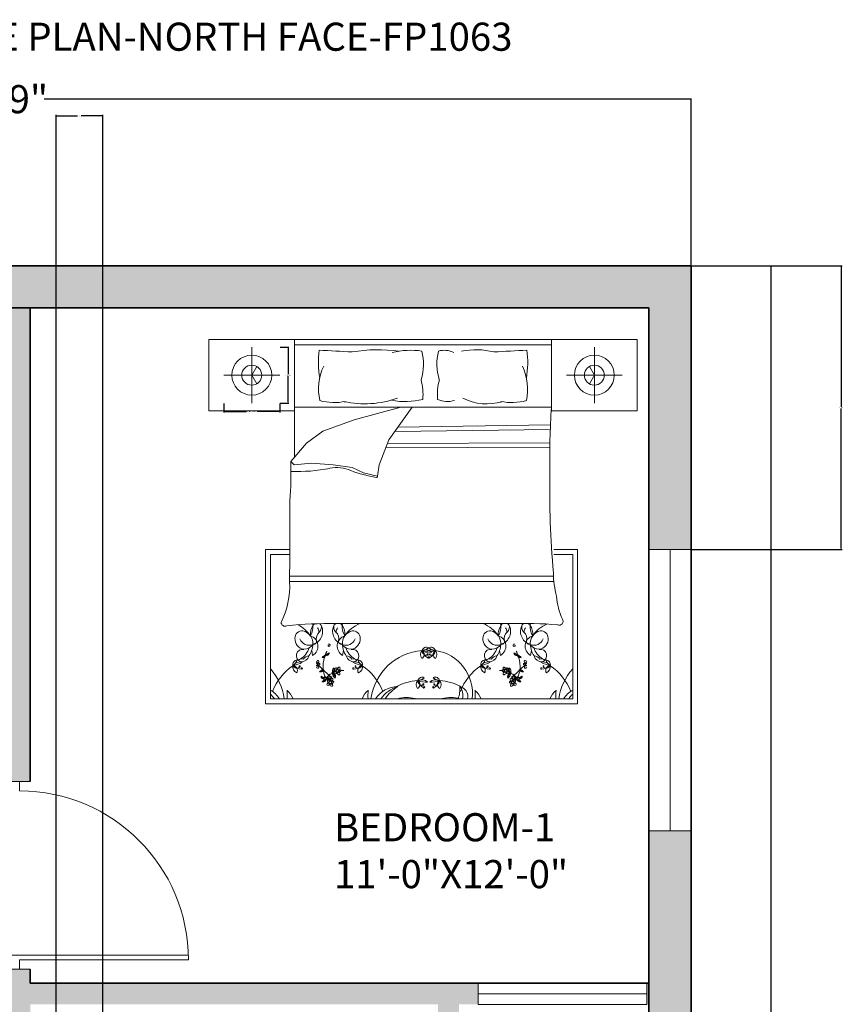
# Model space of a CAD drawing. Units: inches. Extents: x -13 to 349, y -556 to 61.
# Tile 6 of 6: x 174 to 349, y -149 to 61. Entities that reach past the tile are written whole.
import ezdxf

# ---------------------------------------------------------------- set-up
doc = ezdxf.new("R2010")
doc.units = ezdxf.units.IN
doc.header["$MEASUREMENT"] = 0
for name, color, linetype, lineweight in [('A-ANNO-DIMS', 2, 'Continuous', 18), ('A-ANNO-TEXT', 7, 'Continuous', 25), ('A-AREA-IDEN', 7, 'Continuous', 18), ('A-DOOR', 3, 'Continuous', 20), ('A-FURN', 8, 'Continuous', 13), ('A-GLAZ', 5, 'Continuous', 18), ('A-WALL', 7, 'Continuous', 35), ('A-WALL-PATT', 8, 'Continuous', 13)]:
    doc.layers.add(name, color=color, linetype=linetype, lineweight=lineweight)
doc.styles.get("Standard").update_dxf_attribs({"font": 'arial.ttf'})
doc.dimstyles.get("Standard").update_dxf_attribs({"dimtxt": 0.18, "dimasz": 0.18, "dimexe": 0.18, "dimexo": 0.0625, "dimgap": 0.09, "dimtad": 0, "dimtih": 1, "dimtoh": 1, "dimdec": 0, "dimzin": 0, "dimdsep": 46, "dimlunit": 3, "dimtxsty": 'Standard', "dimcen": 0.09, "dimadec": 0, "dimazin": 0, "dimtfac": 1, "dimtdec": 0, "dimtofl": 0, "dimtmove": 0, "dimatfit": 3, "dimfxl": 1, "dimtolj": 1, "dimtzin": 0, "dimarcsym": 0})

# ---------------------------------------------------------------- blocks, each defined once
blk = doc.blocks.new('*D2')
at = {"layer": 'A-ANNO-DIMS', "color": 0, "lineweight": -2, "transparency": 16777216}
for p, q in [((19.76, 8.35), (19.76, 44)), ((19.94, 43.82), (157.81, 43.82)), ((316.58, 43.82), (178.7, 43.82)), ((316.76, 8.35), (316.76, 44))]:
    blk.add_line(p, q, dxfattribs=at)
at = {"layer": 'A-ANNO-DIMS', "color": 0, "transparency": 16777216}
for points in [[(19.94, 43.85), (19.94, 43.79), (19.76, 43.82)], [(316.58, 43.85), (316.58, 43.79), (316.76, 43.82)]]:
    blk.add_solid(points, dxfattribs=at)
at = {"layer": 'Defpoints', "color": 0, "transparency": 16777216}
for p in [(316.76, 43.82), (19.76, 8.29), (316.76, 8.29)]:
    blk.add_point(p, dxfattribs=at)
at = {"layer": 'A-ANNO-DIMS', "color": 0, "transparency": 16777216, "insert": (168.26, 43.82), "char_height": 6, "attachment_point": 5}
blk.add_mtext('\\A1;24\'-9"', dxfattribs=at)
blk = doc.blocks.new('*D3')
at = {"layer": 'A-ANNO-DIMS', "color": 0, "lineweight": -2, "transparency": 16777216}
for p, q in [((316.82, 8.29), (333.9, 8.29)), ((333.72, 8.11), (333.72, -254.62)), ((333.72, -523.53), (333.72, -260.8)), ((316.82, -523.71), (333.9, -523.71))]:
    blk.add_line(p, q, dxfattribs=at)
at = {"layer": 'A-ANNO-DIMS', "color": 0, "transparency": 16777216}
for points in [[(333.69, 8.11), (333.75, 8.11), (333.72, 8.29)], [(333.69, -523.53), (333.75, -523.53), (333.72, -523.71)]]:
    blk.add_solid(points, dxfattribs=at)
at = {"layer": 'Defpoints', "color": 0, "transparency": 16777216}
for p in [(316.76, 8.29), (316.76, -523.71), (333.72, -523.71)]:
    blk.add_point(p, dxfattribs=at)
at = {"layer": 'A-ANNO-DIMS', "color": 0, "transparency": 16777216, "insert": (333.72, -257.71), "char_height": 6, "attachment_point": 5}
blk.add_mtext('\\A1;44\'-4"', dxfattribs=at)
blk = doc.blocks.new('DOOR-SWING-36IN')
for p, q in [((36, 40), (33.75, 40)), ((36, 38), (36, 40)), ((36, 40), (38.25, 40)), ((38.25, 3), (0, 3)), ((36, 2), (0, 2)), ((36, 0), (36, 2)), ((33.75, 0), (38.25, 0))]:
    blk.add_line(p, q)
blk.add_arc((36, 2), 36, 90, 180)
blk = doc.blocks.new('WIN-60IN-D9')
for p, q in [((0, 60), (0, 0)), ((9, 60), (0, 60)), ((4.5, 60), (4.5, 0)), ((9, 0), (9, 60)), ((0, 0), (9, 0))]:
    blk.add_line(p, q)
blk = doc.blocks.new('WIN-36IN-D4_5')
for p, q in [((0, 4.5), (36, 4.5)), ((0, 0), (0, 4.5)), ((36, 4.5), (36, 0)), ((0, 2.25), (36, 2.25)), ((36, 0), (0, 0))]:
    blk.add_line(p, q)
blk = doc.blocks.new('BEDSIDE-LAMP-LG')
for p, q in [((5.97, 0), (5.97, 11.94)), ((0, 5.97), (11.94, 5.97))]:
    blk.add_line(p, q)
for points in [[(5.97, 5.97), (4.91, 7.81)], [(5.97, 5.97), (4.91, 4.12)]]:
    blk.add_lwpolyline(points)
for radius in [4.26, 2.13]:
    blk.add_circle((5.97, 5.97), radius)
blk = doc.blocks.new('*D30')
at = {"layer": 'A-ANNO-DIMS', "color": 0, "lineweight": -2, "transparency": 16777216}
for p, q in [((217.05, -21.06), (217.05, -22.97)), ((217.23, -22.79), (221.89, -22.79)), ((228.81, -22.79), (224.15, -22.79)), ((228.99, -21.06), (228.99, -22.97))]:
    blk.add_line(p, q, dxfattribs=at)
at = {"layer": 'A-ANNO-DIMS', "color": 0, "transparency": 16777216}
for points in [[(217.23, -22.76), (217.23, -22.82), (217.05, -22.79)], [(228.81, -22.76), (228.81, -22.82), (228.99, -22.79)]]:
    blk.add_solid(points, dxfattribs=at)
at = {"layer": 'Defpoints', "color": 0, "transparency": 16777216}
for p in [(217.05, -21), (217.05, -22.79), (228.99, -21)]:
    blk.add_point(p, dxfattribs=at)
at = {"layer": 'A-ANNO-DIMS', "color": 0, "transparency": 16777216, "insert": (223.02, -22.79), "char_height": 0.18, "attachment_point": 5}
blk.add_mtext('\\A1;LAMP A 1\'-0" TYP.', dxfattribs=at)
blk = doc.blocks.new('*D31')
at = {"layer": 'A-ANNO-DIMS', "color": 0, "lineweight": -2, "transparency": 16777216}
for p, q in [((229.05, -9.06), (230.96, -9.06)), ((230.78, -9.24), (230.78, -14.85)), ((230.78, -20.82), (230.78, -15.21)), ((229.05, -21), (230.96, -21))]:
    blk.add_line(p, q, dxfattribs=at)
at = {"layer": 'A-ANNO-DIMS', "color": 0, "transparency": 16777216}
for points in [[(230.75, -9.24), (230.81, -9.24), (230.78, -9.06)], [(230.75, -20.82), (230.81, -20.82), (230.78, -21)]]:
    blk.add_solid(points, dxfattribs=at)
at = {"layer": 'Defpoints', "color": 0, "transparency": 16777216}
for p in [(228.99, -9.06), (228.99, -21), (230.78, -21)]:
    blk.add_point(p, dxfattribs=at)
at = {"layer": 'A-ANNO-DIMS', "color": 0, "transparency": 16777216, "insert": (230.78, -15.03), "char_height": 0.18, "attachment_point": 5}
blk.add_mtext('\\A1;1\'-0" TYP.', dxfattribs=at)
blk = doc.blocks.new('*D37')
at = {"layer": 'A-ANNO-DIMS', "color": 0, "lineweight": -2, "transparency": 16777216}
for p, q in [((181.26, -353.65), (181.26, 40.47)), ((181.44, 40.29), (185.86, 40.29)), ((191.08, 40.29), (186.65, 40.29)), ((191.26, -353.65), (191.26, 40.47))]:
    blk.add_line(p, q, dxfattribs=at)
at = {"layer": 'A-ANNO-DIMS', "color": 0, "transparency": 16777216}
for points in [[(181.44, 40.32), (181.44, 40.26), (181.26, 40.29)], [(191.08, 40.32), (191.08, 40.26), (191.26, 40.29)]]:
    blk.add_solid(points, dxfattribs=at)
at = {"layer": 'Defpoints', "color": 0, "transparency": 16777216}
for p in [(191.26, 40.29), (181.26, -353.71), (191.26, -353.71)]:
    blk.add_point(p, dxfattribs=at)
at = {"layer": 'A-ANNO-DIMS', "color": 0, "transparency": 16777216, "insert": (186.26, 40.29), "char_height": 0.18, "attachment_point": 5}
blk.add_mtext('\\A1;0\'-10"', dxfattribs=at)
blk = doc.blocks.new('*D41')
at = {"layer": 'A-ANNO-DIMS', "color": 0, "lineweight": -2, "transparency": 16777216}
for p, q in [((316.82, 8.29), (348.94, 8.29)), ((348.76, 8.11), (348.76, -21.77)), ((348.76, -52.01), (348.76, -22.13)), ((316.82, -52.19), (348.94, -52.19))]:
    blk.add_line(p, q, dxfattribs=at)
at = {"layer": 'A-ANNO-DIMS', "color": 0, "transparency": 16777216}
for points in [[(348.73, 8.11), (348.79, 8.11), (348.76, 8.29)], [(348.73, -52.01), (348.79, -52.01), (348.76, -52.19)]]:
    blk.add_solid(points, dxfattribs=at)
at = {"layer": 'Defpoints', "color": 0, "transparency": 16777216}
for p in [(316.76, 8.29), (316.76, -52.19), (348.76, -52.19)]:
    blk.add_point(p, dxfattribs=at)
at = {"layer": 'A-ANNO-DIMS', "color": 0, "transparency": 16777216, "insert": (348.76, -21.95), "char_height": 0.18, "attachment_point": 5}
blk.add_mtext('\\A1;5\'-0 1/2"', dxfattribs=at)

msp = doc.modelspace()

# ---------------------------------------------------------------- hatches: boundary and pattern name
at = {"layer": 'A-WALL-PATT'}
h = msp.add_hatch(color=256, dxfattribs=at)
h.dxf.hatch_style = 1
h.paths.add_polyline_path([(316.76, 8.29), (171.26, 8.29), (171.26, -0.71), (307.76, -0.71), (307.76, -52.19), (316.76, -52.19)])
h.paths.add_polyline_path([(175.76, -0.71), (171.26, -0.71), (171.26, -82.21), (165.24, -82.21), (165.24, -86.71), (171.26, -86.71), (171.26, -101.71), (173.51, -101.71), (175.76, -101.71)])
h.paths.add_polyline_path([(171.26, -25.21), (165.17, -25.21), (165.17, -34.21), (171.26, -34.21)])
h.paths.add_polyline_path([(141.17, -25.21), (127.76, -25.21), (127.76, -34.21), (141.17, -34.21)])
h.paths.add_polyline_path([(28.76, -25.21), (24.26, -25.21), (19.76, -25.21), (19.76, -78.88), (28.76, -78.88)])
h.paths.add_polyline_path([(99.76, -29.71), (99.76, -25.21), (28.76, -25.21), (28.76, -34.21), (99.76, -34.21)])
h.paths.add_polyline_path([(135.26, -86.71), (143.68, -86.71), (143.68, -82.21), (135.26, -82.21), (135.26, -34.21), (130.76, -34.21), (130.76, -101.71), (133.01, -101.71), (135.26, -101.71)])
h.paths.add_polyline_path([(135.26, -141.71), (130.76, -141.71), (130.76, -144.71), (28.76, -144.71), (28.76, -149.21), (135.26, -149.21)])
h.paths.add_polyline_path([(28.76, -138.88), (19.76, -138.88), (19.76, -156.62), (28.76, -156.62)])
h.paths.add_polyline_path([(28.76, -192.62), (19.76, -192.62), (19.76, -271.06), (28.76, -271.06)])
h.paths.add_polyline_path([(28.76, -307.06), (19.76, -307.06), (19.76, -385.56), (28.76, -385.56)])
h.paths.add_polyline_path([(28.76, -445.56), (19.76, -445.56), (19.76, -523.71), (28.76, -523.71)])
h.paths.add_polyline_path([(307.76, -431.71), (261.76, -431.71), (261.76, -353.71), (264.76, -353.71), (264.76, -349.21), (175.76, -349.21), (175.76, -248.21), (173.51, -248.21), (171.26, -248.21), (171.26, -317.21), (168.26, -317.21), (168.26, -321.71), (171.26, -321.71), (171.26, -353.71), (257.26, -353.71), (257.26, -431.71), (171.26, -431.71), (171.26, -436.21), (307.76, -436.21)])
h.paths.add_polyline_path([(316.76, -424.85), (307.76, -424.85), (307.76, -436.21), (316.76, -436.21)])
h.paths.add_polyline_path([(316.76, -305.84), (307.76, -305.84), (307.76, -400.85), (316.76, -400.85)])
h.paths.add_polyline_path([(307.76, -349.21), (292.76, -349.21), (292.76, -351.46), (292.76, -353.71), (307.76, -353.71)], flags=17)
h.paths.add_polyline_path([(271.19, -200.71), (267.26, -200.71), (267.26, -186.96), (262.76, -186.96), (262.76, -200.71), (175.76, -200.71), (175.76, -180.21), (173.51, -180.21), (171.26, -180.21), (171.26, -208.21), (175.76, -208.21), (175.76, -205.21), (271.19, -205.21)])
h.paths.add_polyline_path([(316.76, -112.19), (307.76, -112.19), (307.76, -245.84), (316.76, -245.84)])
h.paths.add_polyline_path([(271.33, -144.71), (175.76, -144.71), (175.76, -141.71), (171.26, -141.71), (171.26, -152.21), (175.76, -152.21), (175.76, -149.21), (262.76, -149.21), (262.76, -162.96), (267.26, -162.96), (267.26, -149.21), (271.33, -149.21)])
h.paths.add_polyline_path([(307.76, -200.71), (307.19, -200.71), (307.19, -205.21), (307.76, -205.21)])
h.paths.add_polyline_path([(307.76, -144.71), (307.33, -144.71), (307.33, -149.21), (307.76, -149.21)])

# ---------------------------------------------------------------- linework, layer by layer
at = {"layer": 'A-FURN'}
for p, q in [((213.88, -7.42), (305.24, -7.42)), ((232.15, -7.42), (232.15, -32.49)), ((286.97, -8.59), (232.15, -8.59)), ((232.15, -21.85), (286.97, -21.85)), ((244.84, -24.57), (254.81, -21.85)), ((257.25, -21.85), (252.24, -28.82)), ((238.18, -26.97), (244.84, -24.57)), ((234.67, -29.56), (238.18, -26.97)), ((286.69, -26.59), (253.51, -27.06)), ((286.72, -25.65), (254.2, -26.11)), ((252.24, -28.82), (250.21, -34.19)), ((231.34, -33.45), (234.67, -29.56)), ((286.64, -30.4), (251.59, -30.55)), ((286.64, -29.46), (251.95, -29.6)), ((232.08, -34.19), (231.34, -33.45)), ((235.78, -33.82), (232.08, -34.19)), ((240.4, -34.19), (235.78, -33.82)), ((244.47, -34.74), (240.4, -34.19)), ((246.88, -35.85), (244.47, -34.74)), ((250.21, -34.19), (249.84, -36.59)), ((249.84, -36.59), (246.88, -35.85)), ((225.94, -52.2), (231.11, -52.2)), ((225.94, -85.11), (225.94, -52.2)), ((287.48, -52.2), (292.54, -52.2)), ((292.54, -52.2), (292.54, -85.11)), ((231.11, -53.26), (227, -53.26)), ((227, -53.26), (227, -84.05)), ((291.48, -53.26), (287.46, -53.26)), ((291.48, -84.05), (291.48, -53.26)), ((287.38, -57.9), (231.1, -57.9)), ((287.47, -59.04), (231.1, -59.04)), ((278.11, -68.01), (241.01, -68.01)), ((236, -74.79), (235.8, -73.76)), ((242.39, -74.79), (242.59, -73.76)), ((276.1, -74.79), (275.89, -73.76)), ((282.48, -74.79), (282.68, -73.76)), ((292.54, -85.11), (225.94, -85.11)), ((227, -84.05), (291.48, -84.05))]:
    msp.add_line(p, q, dxfattribs=at)
for points in [[(232.15, -22.64), (213.88, -22.64), (213.88, -7.42)], [(286.97, -7.42), (286.97, -22.64), (305.24, -22.64), (305.24, -7.42)]]:
    msp.add_lwpolyline(points, dxfattribs=at)
for points in [[(237.4, -9.7, 0.074897), (237.51, -15.66, -0.472817)], [(259.13, -16, 0.14099), (259.31, -9.91, 0.235245)], [(263.03, -16, -0.14099), (262.85, -9.91, -0.235245)], [(281.72, -9.7, -0.074897), (281.61, -15.66, 0.472817)], [(231.15, -41.81, 0.001242), (231.1, -59.14, -0.127202), (229.27, -67.78)], [(287.36, -57.18, 0.056112), (288.02, -62.2, 0.095341), (289.3, -67.05)]]:
    msp.add_lwpolyline(points, format="xyb", dxfattribs=at)
for centre in [(241.28, -78.1), (277.2, -78.1), (239.76, -80.55), (278.72, -80.55)]:
    msp.add_circle(centre, 0.233, dxfattribs=at)
for centre, radius, start, end in [((287.75, 859.68), 870.84, 266.68521, 267.14978), ((249.92, -42.75), 33.13, 82.2196, 99.497), ((256.92, -26.01), 16.28, 81.5249, 103.96), ((264.1, -14.25), 4.52, 63.3437, 106.1026), ((270.88, -25.68), 16.06, 76.3427, 101.1841), ((231.37, 859.68), 870.84, 272.85022, 273.31479), ((249.04, -18.06), 11.77, 155.1316, 191.7583), ((270.08, -18.06), 11.77, 348.2417, 24.8684), ((248.36, -19.05), 11.19, 354.0129, 15.8293), ((273.8, -19.05), 11.19, 164.1707, 185.9871), ((240.66, -8.63), 12.24, 255.1039, 281.0369), ((247.1, 0.08), 21.23, 258.0397, 289.2615), ((255.7, -4.56), 16.11, 259.8617, 283.6238), ((264.72, -15.83), 4.84, 245.0183, 288.5407), ((273.18, -9.53), 11.63, 243.8761, 286.1746), ((278.46, -8.63), 12.24, 258.9631, 284.8961), ((450.73, -33.02), 164.15, 176.1, 180.9282), ((147.58, -35.72), 83.79, 355.8294, 1.553), ((232.9, -1.1), 34.48, 267.4519, 281.3392), ((241.14, -42.19), 7.44, 66.2616, 101.3392), ((256.18, -2.07), 35.43, 250.1194, 259.3383), ((500.7, -38.99), 214.12, 179.1145, 184.8735), ((249.63, -36.66), 0.22, 268.8623, 19.7536), ((288.61, -67.51), 0.833, 246.5219, 33.8264), ((230.11, -67.72), 0.843, 183.98, 297.3412), ((239.92, -163.1), 95.1, 89.3433, 95.6887), ((229.75, -74.44), 6.91, 33.6671, 63.2997), ((239.02, -70.33), 3.52, 145.785, 184.7304), ((232.29, -68.69), 3.78, 328.8218, 9.1554), ((236.98, -69.02), 1.1, 120.0293, 142.325), ((235.22, -69.67), 2.91, 289.2822, 29.1751), ((234.78, -70.2), 2.63, 7.436, 29.9149), ((236.51, -68.8), 1.37, 311.5653, 23.8354), ((236.98, -69.02), 1.1, 44.4517, 63.558), ((243.17, -69.67), 2.91, 150.8249, 250.7178), ((241.88, -68.8), 1.37, 156.1646, 228.4347), ((241.41, -69.02), 1.1, 113.229, 135.5483), ((243.61, -70.2), 2.63, 150.0851, 172.564), ((241.41, -69.02), 1.1, 37.675, 66.7144), ((239.37, -70.33), 3.52, 355.2696, 34.215), ((246.1, -68.69), 3.78, 169.7133, 211.1782), ((248.63, -74.44), 6.91, 111.4941, 146.3329), ((269.85, -74.44), 6.91, 33.6671, 68.5059), ((279.11, -70.33), 3.52, 145.785, 184.7304), ((272.38, -68.69), 3.78, 328.8218, 10.2867), ((277.07, -69.02), 1.1, 113.2856, 142.325), ((275.32, -69.67), 2.91, 289.2822, 29.1751), ((274.88, -70.2), 2.63, 7.436, 29.9149), ((277.07, -69.02), 1.1, 44.4517, 66.7144), ((276.61, -68.8), 1.37, 311.5653, 23.8354), ((280.9, -156.86), 88.89, 85.2402, 91.8035), ((283.26, -69.67), 2.91, 150.8249, 250.7178), ((281.97, -68.8), 1.37, 156.1646, 228.4347), ((281.5, -69.02), 1.1, 106.6343, 135.5483), ((283.7, -70.2), 2.63, 150.0851, 172.564), ((281.5, -69.02), 1.1, 37.675, 72.5814), ((279.46, -70.33), 3.52, 355.2696, 34.215), ((286.19, -68.69), 3.78, 169.249, 211.1782), ((288.73, -74.44), 6.91, 113.6453, 146.3329), ((234.41, -71.34), 2.18, 174.9449, 262.8857), ((233.78, -71.12), 1.54, 84.4856, 181.0538), ((235.27, -70.52), 2.12, 201.5819, 291.4221), ((233.31, -72.26), 2.75, 355.2933, 76.921), ((234.87, -72.82), 2.27, 299.9085, 73.1337), ((238.66, -71.23), 1.87, 131.5653, 195.1471), ((239.73, -71.23), 1.87, 344.8529, 48.4347), ((243.52, -72.82), 2.27, 106.8663, 240.0915), ((245.08, -72.26), 2.75, 103.079, 184.7067), ((243.12, -70.52), 2.12, 248.5779, 338.4181), ((243.97, -71.34), 2.18, 277.1143, 5.0551), ((244.61, -71.12), 1.54, 358.9462, 95.5144), ((273.88, -71.12), 1.54, 84.4856, 181.0538), ((274.51, -71.34), 2.18, 174.9449, 262.8857), ((275.37, -70.52), 2.12, 201.5819, 291.4221), ((273.4, -72.26), 2.75, 355.2933, 76.921), ((274.96, -72.82), 2.27, 299.9085, 73.1337), ((278.76, -71.23), 1.87, 131.5653, 195.1471), ((279.82, -71.23), 1.87, 344.8529, 48.4347), ((283.61, -72.82), 2.27, 106.8663, 240.0915), ((285.17, -72.26), 2.75, 103.079, 184.7067), ((283.21, -70.52), 2.12, 248.5779, 338.4181), ((284.07, -71.34), 2.18, 277.1143, 5.0551), ((284.7, -71.12), 1.54, 358.9462, 95.5144), ((233.91, -74.86), 1.37, 80.264, 250.8688), ((231.19, -71.84), 4.31, 301.2614, 341.7045), ((234.04, -70.86), 2.65, 272.3591, 324.0401), ((231.15, -72.19), 4.9, 326.2883, 356.5076), ((239.02, -70.33), 3.52, 212.7011, 216.3445), ((236.31, -71.86), 0.567, 257.3041, 15.1471), ((239.46, -72.72), 0.176, 102.7051, 280.4384), ((239.44, -72.62), 0.286, 280.4384, 100.4136), ((242.08, -71.86), 0.567, 164.8529, 282.6959), ((239.37, -70.33), 3.52, 323.6555, 327.2989), ((244.35, -70.86), 2.65, 215.9599, 267.6409), ((247.23, -72.19), 4.9, 183.4924, 213.7117), ((247.19, -71.84), 4.31, 198.2955, 238.7386), ((244.48, -74.86), 1.37, 289.1312, 99.736), ((260.29, -74.04), 0.989, 63.0274, 163.8037), ((259.29, -71.73), 2.04, 271.4585, 315.3727), ((261.24, -74.04), 0.989, 16.1963, 116.9726), ((262.24, -71.73), 2.04, 224.6273, 268.5415), ((274.01, -74.86), 1.37, 80.264, 250.8688), ((271.29, -71.84), 4.31, 301.2614, 341.7045), ((274.13, -70.86), 2.65, 272.3591, 324.0401), ((271.25, -72.19), 4.9, 326.2883, 356.5076), ((279.11, -70.33), 3.52, 212.7011, 216.3445), ((276.4, -71.86), 0.567, 257.3041, 15.1471), ((279.05, -72.62), 0.286, 79.5864, 259.5616), ((279.03, -72.72), 0.176, 259.5616, 77.2949), ((282.17, -71.86), 0.567, 164.8529, 282.6959), ((279.46, -70.33), 3.52, 323.6555, 327.2989), ((284.45, -70.86), 2.65, 215.9599, 267.6409), ((287.33, -72.19), 4.9, 183.4924, 213.7117), ((287.29, -71.84), 4.31, 198.2955, 238.7386), ((284.57, -74.86), 1.37, 289.1312, 99.736), ((233.63, -76.35), 0.84, 63.9755, 143.2681), ((233.58, -74.45), 1.71, 265.969, 344.3045), ((235.43, -76.73), 1.82, 96.1662, 141.5825), ((238.45, -75.45), 0.48, 101.3256, 154.4621), ((237.76, -73.82), 1.44, 280.2588, 300.656), ((238.09, -72.66), 2.58, 268.3264, 277.1302), ((245.79, -77.32), 7.57, 163.5842, 183.8277), ((237.45, -73.82), 1.47, 308.2101, 316.3071), ((238.35, -74.79), 0.438, 278.3432, 4.2869), ((238.1, -74.4), 0.766, 300.656, 332.6341), ((238.68, -74.91), 0.186, 55.7657, 157.4417), ((245.79, -77.32), 7.57, 153.0032, 159.8941), ((238.97, -74.73), 0.186, 84.3784, 186.0543), ((238.79, -73.99), 0.766, 269.1859, 301.164), ((239.02, -74.38), 0.438, 237.5332, 323.4768), ((238.59, -73.13), 1.47, 285.5129, 293.6099), ((239.55, -74.78), 0.48, 87.3579, 140.4944), ((238.44, -73.41), 1.44, 301.164, 321.5612), ((237.27, -73.16), 2.58, 324.6898, 333.4936), ((242.96, -76.73), 1.82, 38.4175, 83.8338), ((244.81, -74.45), 1.71, 195.6955, 274.031), ((244.76, -76.35), 0.84, 36.7319, 116.0245), ((260.27, -85.66), 11.93, 94.4623, 172.255), ((260.32, -74.65), 1.32, 137.7873, 219.1145), ((258.82, -74.61), 0.996, 298.5391, 58.3627), ((260.12, -75.48), 1.89, 45.5411, 114.3101), ((261.84, -65.8), 8.35, 252.593, 267.2582), ((260.32, -73.8), 0.976, 177.7585, 283.852), ((262.2, -72.79), 3.02, 198.9159, 238.011), ((261.41, -75.48), 1.89, 65.6899, 134.4589), ((259.69, -65.8), 8.35, 272.7418, 287.407), ((260.52, -74.62), 0.129, 283.852, 219.9245), ((260.68, -75.22), 0.148, 238.011, 71.5592), ((260.7, -75.15), 0.072, 71.5592, 188.0167), ((260.85, -75.22), 0.148, 108.4408, 301.989), ((260.83, -75.15), 0.072, 351.9833, 108.4408), ((261, -74.57), 0.0778, 320.1909, 256.0209), ((259.33, -72.79), 3.02, 301.989, 341.0841), ((261.21, -73.8), 0.976, 256.148, 2.2415), ((262.71, -74.61), 0.996, 121.6373, 241.4609), ((261.21, -74.65), 1.32, 320.8855, 42.2127), ((260.87, -82.9), 9.23, 352.8636, 81.8197), ((273.72, -76.35), 0.84, 63.9755, 143.2681), ((273.68, -74.45), 1.71, 265.969, 344.3045), ((275.52, -76.73), 1.82, 96.1662, 141.5825), ((280.04, -73.41), 1.44, 218.4388, 238.836), ((278.93, -74.78), 0.48, 39.5056, 92.6421), ((281.21, -73.16), 2.58, 206.5064, 215.3102), ((279.46, -74.38), 0.438, 216.5232, 302.4668), ((279.69, -73.99), 0.766, 238.836, 270.8141), ((279.89, -73.13), 1.47, 246.3901, 254.4871), ((272.69, -77.32), 7.57, 20.1059, 26.9968), ((279.51, -74.73), 0.186, 353.9457, 95.6216), ((279.8, -74.91), 0.186, 22.5583, 124.2343), ((280.14, -74.79), 0.438, 175.7131, 261.6568), ((280.38, -74.4), 0.766, 207.3659, 239.344), ((272.69, -77.32), 7.57, 356.1723, 16.4158), ((281.04, -73.82), 1.47, 223.6929, 231.7899), ((280.72, -73.82), 1.44, 239.344, 259.7412), ((280.39, -72.66), 2.58, 262.8698, 271.6736), ((280.03, -75.45), 0.48, 25.5379, 78.6744), ((284.9, -74.45), 1.71, 195.6955, 274.031), ((283.05, -76.73), 1.82, 38.4175, 83.8338), ((284.85, -76.35), 0.84, 36.7319, 116.0245), ((218.12, -85.66), 11.93, 7.745, 41.8856), ((238.53, -86.84), 11.93, 124.3865, 158.5908), ((232.75, -76.76), 0.989, 92.9516, 193.728), ((233.08, -77.27), 1.32, 167.7115, 249.0387), ((230.73, -75.25), 2.04, 301.3827, 345.2969), ((233.32, -78.09), 1.89, 75.4653, 144.2343), ((229.98, -68.84), 8.35, 282.5173, 297.1824), ((231.76, -77.99), 0.996, 328.4633, 88.2869), ((233.78, -74.72), 3.02, 228.8402, 267.9352), ((232.65, -76.54), 0.976, 207.6827, 313.7762), ((233.24, -77.15), 0.129, 313.7762, 249.7183), ((233.66, -77.51), 0.072, 101.4834, 217.9409), ((233.67, -77.59), 0.148, 267.9352, 101.4834), ((237.09, -76.36), 0.388, 101.5637, 142.6358), ((236.77, -76.72), 0.233, 273.2768, 86.7232), ((237.09, -77.15), 0.384, 217.7621, 259.0403), ((237.04, -76.5), 0.222, 91.1081, 181.8675), ((237.5, -76.63), 0.706, 203.4276, 227.6104), ((237.28, -76.94), 0.481, 80.3487, 133.6538), ((237.19, -76.54), 0.381, 229.7889, 317.6792), ((236.78, -76.05), 0.559, 288.7263, 352.5032), ((236.76, -77.35), 0.541, 355.053, 68.3618), ((237.19, -77.44), 0.762, 83.0852, 105.7171), ((237.16, -76.08), 0.18, 345.2356, 144.9248), ((237.12, -77.38), 0.178, 232.4737, 355.053), ((231.91, -83.76), 8.67, 43.1541, 52.0459), ((237.32, -76.67), 0.2, 317.6792, 80.3487), ((239.5, -77.75), 1.06, 304.5369, 16.3699), ((240.97, -78.05), 0.75, 127.3105, 187.9252), ((239.94, -77.97), 0.771, 355.0106, 41.658), ((241.02, -77.77), 0.317, 126.1046, 271.4281), ((240.99, -77.69), 0.228, 353.7526, 131.7054), ((240.77, -77.96), 0.32, 0.0645, 61.1507), ((241.6, -77.74), 0.388, 101.5637, 176.365), ((241.55, -77.88), 0.222, 91.1081, 181.8675), ((241.29, -77.43), 0.559, 288.7263, 352.5032), ((241.67, -77.46), 0.18, 345.2356, 144.9248), ((244.72, -77.59), 0.148, 78.5166, 272.0648), ((245.07, -78.09), 1.89, 35.7657, 104.5347), ((248.41, -68.84), 8.35, 242.8176, 257.4827), ((244.61, -74.72), 3.02, 272.0648, 311.1598), ((244.73, -77.51), 0.072, 322.0591, 78.5166), ((245.73, -76.54), 0.976, 226.2238, 332.3173), ((245.16, -77.1), 0.0778, 290.2667, 226.2271), ((246.63, -77.99), 0.996, 91.7131, 211.5367), ((245.64, -76.76), 0.989, 346.272, 87.0484), ((247.66, -75.25), 2.04, 194.7031, 238.6173), ((245.31, -77.27), 1.32, 290.9613, 12.2885), ((239.86, -86.84), 11.93, 21.4092, 55.6135), ((278.62, -86.84), 11.93, 124.3865, 158.5908), ((273.18, -77.27), 1.32, 167.7115, 249.0387), ((272.85, -76.76), 0.989, 92.9516, 193.728), ((270.82, -75.25), 2.04, 301.3827, 345.2969), ((273.41, -78.09), 1.89, 75.4653, 144.2343), ((270.08, -68.84), 8.35, 282.5173, 297.1824), ((272.75, -76.54), 0.976, 207.6827, 313.7762), ((273.87, -74.72), 3.02, 228.8402, 267.9352), ((271.85, -77.99), 0.996, 328.4633, 88.2869), ((273.33, -77.15), 0.129, 313.7762, 249.7183), ((273.75, -77.51), 0.072, 101.4834, 217.9409), ((273.77, -77.59), 0.148, 267.9352, 101.4834), ((276.81, -77.46), 0.18, 35.0752, 194.7644), ((277.19, -77.43), 0.559, 187.4968, 251.2737), ((276.93, -77.88), 0.222, 358.1325, 88.8919), ((276.88, -77.74), 0.388, 3.635, 78.4363), ((277.49, -77.69), 0.228, 48.2946, 186.2474), ((277.71, -77.96), 0.32, 118.8493, 179.9355), ((277.46, -77.77), 0.317, 268.5719, 53.8954), ((278.54, -77.97), 0.771, 138.342, 184.9894), ((278.98, -77.75), 1.06, 163.6301, 235.4631), ((277.51, -78.05), 0.75, 352.0748, 52.6895), ((286.57, -83.76), 8.67, 127.9541, 136.8459), ((281.16, -76.67), 0.2, 99.6513, 222.3208), ((281.29, -76.54), 0.381, 222.3208, 310.2111), ((281.21, -76.94), 0.481, 46.3462, 99.6513), ((281.32, -76.08), 0.18, 35.0752, 194.7644), ((281.7, -76.05), 0.559, 187.4968, 251.2737), ((281.72, -77.35), 0.541, 111.6382, 184.947), ((281.36, -77.38), 0.178, 184.947, 307.5263), ((281.3, -77.44), 0.762, 74.2829, 96.9148), ((281.44, -76.5), 0.222, 358.1325, 88.8919), ((280.98, -76.63), 0.706, 312.3896, 336.5724), ((281.39, -76.36), 0.388, 37.3642, 78.4363), ((281.4, -77.15), 0.384, 280.9597, 322.2379), ((281.71, -76.72), 0.233, 93.2768, 266.7232), ((284.81, -77.59), 0.148, 78.5166, 272.0648), ((285.16, -78.09), 1.89, 35.7657, 104.5347), ((288.5, -68.84), 8.35, 242.8176, 257.4827), ((284.71, -74.72), 3.02, 272.0648, 311.1598), ((284.83, -77.51), 0.072, 322.0591, 78.5166), ((285.83, -76.54), 0.976, 226.2238, 332.3173), ((285.26, -77.1), 0.0778, 290.2667, 226.2271), ((286.72, -77.99), 0.996, 91.7131, 211.5367), ((287.75, -75.25), 2.04, 194.7031, 238.6173), ((285.73, -76.76), 0.989, 346.272, 87.0484), ((285.4, -77.27), 1.32, 290.9613, 12.2885), ((279.95, -86.84), 11.93, 21.4092, 55.6135), ((300.36, -85.66), 11.93, 138.1144, 172.255), ((237.9, -78.52), 0.48, 101.3256, 154.4621), ((237.21, -76.89), 1.44, 280.2588, 300.656), ((237.55, -75.74), 2.58, 268.3264, 277.1302), ((236.9, -76.9), 1.47, 308.2101, 316.3071), ((238.07, -79.36), 0.26, 146.8636, 236.9021), ((241.73, -73.64), 6.8, 235.1882, 238.8844), ((238.51, -78.98), 0.703, 199.4799, 267.6828), ((237.8, -77.86), 0.438, 278.3432, 4.2869), ((238.43, -79.25), 0.606, 212.8155, 277.3992), ((237.56, -77.48), 0.766, 300.656, 332.6341), ((238.13, -77.98), 0.186, 55.7657, 157.4417), ((238.35, -79.23), 0.269, 238.8844, 314.2646), ((242.02, -77.51), 3.79, 184.756, 209.2041), ((247.48, -69.44), 12.48, 222.2412, 232.1744), ((238.3, -79.83), 0.606, 280.3057, 17.1958), ((238.24, -79.89), 0.269, 306.3746, 21.7548), ((238.68, -79.72), 0.203, 19.3605, 201.7548), ((238.68, -79.57), 0.203, 311.8703, 134.2646), ((242.5, -81.41), 4.05, 153.7819, 158.2913), ((239.27, -78.65), 1.06, 247.2305, 319.0635), ((238.92, -79), 0.624, 264.4544, 310.6188), ((242.02, -77.51), 3.79, 214.0033, 222.4917), ((239.38, -79.25), 0.645, 218.3208, 298.8162), ((242.41, -82.55), 4.55, 120.544, 139.818), ((239.82, -80.05), 0.75, 70.0041, 130.6188), ((239.33, -79.13), 0.771, 297.7043, 344.3516), ((240.15, -79.91), 0.18, 345.2356, 144.9248), ((240.07, -77.99), 0.645, 272.8499, 356.1226), ((239.61, -78.24), 0.624, 321.7607, 7.9252), ((239.74, -79.14), 0.624, 8.7227, 54.8872), ((239.77, -79.64), 1.06, 0.278, 72.111), ((240.25, -79.25), 0.645, 20.5253, 88.5375), ((241.1, -78.93), 0.75, 188.7227, 249.3375), ((240.79, -78.53), 0.23, 148.0499, 225.6268), ((242.41, -82.55), 4.55, 113.0501, 113.8477), ((241.22, -78.8), 0.733, 104.7558, 148.0499), ((240.81, -78.28), 0.459, 247.4086, 351.4386), ((240.14, -79.3), 0.771, 334.9899, 21.6373), ((240.94, -78.29), 0.154, 262.906, 7.132), ((240.85, -77.69), 0.366, 311.8413, 355.7877), ((241.6, -78.53), 0.384, 151.2196, 259.0403), ((242.01, -78.02), 0.706, 203.4276, 227.6104), ((241.79, -78.32), 0.481, 80.3487, 133.6538), ((241.7, -77.93), 0.381, 229.7889, 317.6792), ((241.27, -78.73), 0.541, 355.053, 68.3618), ((241.7, -78.82), 0.762, 83.0852, 105.7171), ((241.63, -78.76), 0.178, 232.4737, 355.053), ((241.83, -78.05), 0.2, 317.6792, 80.3487), ((242.41, -82.55), 4.55, 87.1071, 94.7585), ((259.38, -80.43), 0.989, 63.0274, 163.8037), ((258.38, -78.12), 2.04, 271.4585, 315.3727), ((262.15, -80.43), 0.989, 16.1963, 116.9726), ((263.15, -78.12), 2.04, 224.6273, 268.5415), ((276.07, -82.55), 4.55, 85.2415, 92.8929), ((276.65, -78.05), 0.2, 99.6513, 222.3208), ((276.78, -77.93), 0.381, 222.3208, 310.2111), ((276.7, -78.32), 0.481, 46.3462, 99.6513), ((277.21, -78.73), 0.541, 111.6382, 184.947), ((276.85, -78.76), 0.178, 184.947, 307.5263), ((276.79, -78.82), 0.762, 74.2829, 96.9148), ((276.47, -78.02), 0.706, 312.3896, 336.5724), ((276.89, -78.53), 0.384, 280.9597, 28.7804), ((277.68, -78.28), 0.459, 188.5614, 292.5914), ((277.63, -77.69), 0.366, 184.2123, 228.1587), ((277.55, -78.29), 0.154, 172.868, 277.094), ((277.26, -78.8), 0.733, 31.9501, 75.2442), ((278.35, -79.3), 0.771, 158.3627, 205.0101), ((278.23, -79.25), 0.645, 91.4625, 159.4747), ((278.71, -79.64), 1.06, 107.889, 179.722), ((277.38, -78.93), 0.75, 290.6625, 351.2773), ((278.42, -77.99), 0.645, 183.8774, 267.1501), ((276.07, -82.55), 4.55, 66.1523, 66.9499), ((277.69, -78.53), 0.23, 314.3732, 31.9501), ((278.74, -79.14), 0.624, 125.1128, 171.2773), ((278.33, -79.91), 0.18, 35.0752, 194.7644), ((278.87, -78.24), 0.624, 172.0748, 218.2393), ((276.07, -82.55), 4.55, 40.182, 59.456), ((278.66, -80.05), 0.75, 49.3812, 109.9959), ((279.21, -78.65), 1.06, 220.9365, 292.7695), ((279.15, -79.13), 0.771, 195.6484, 242.2957), ((271, -69.44), 12.48, 307.8256, 317.7588), ((279.1, -79.25), 0.645, 241.1838, 321.6792), ((279.56, -79), 0.624, 229.3812, 275.5456), ((276.46, -77.51), 3.79, 317.5083, 325.9967), ((280.19, -79.83), 0.606, 162.8042, 259.6943), ((279.8, -79.57), 0.203, 45.7354, 228.1297), ((279.8, -79.72), 0.203, 338.2452, 160.6395), ((275.98, -81.41), 4.05, 21.7087, 26.2181), ((276.46, -77.51), 3.79, 330.7959, 355.244), ((280.13, -79.23), 0.269, 225.7354, 301.1156), ((280.05, -79.25), 0.606, 262.6008, 327.1845), ((280.24, -79.89), 0.269, 158.2452, 233.6254), ((279.97, -78.98), 0.703, 272.3172, 340.5201), ((280.35, -77.98), 0.186, 22.5583, 124.2343), ((280.68, -77.86), 0.438, 175.7131, 261.6568), ((280.92, -77.48), 0.766, 207.3659, 239.344), ((276.75, -73.64), 6.8, 301.1156, 304.8118), ((281.58, -76.9), 1.47, 223.6929, 231.7899), ((281.27, -76.89), 1.44, 239.344, 259.7412), ((280.42, -79.36), 0.26, 303.0979, 33.1364), ((280.94, -75.74), 2.58, 262.8698, 271.6736), ((280.58, -78.52), 0.48, 25.5379, 78.6744), ((238.08, -79.66), 0.703, 266.9701, 338.2913), ((234.37, -74.64), 6.8, 302.6784, 306.3746), ((238.26, -80.21), 0.26, 214.3538, 304.3923), ((239.27, -80.99), 0.23, 148.0499, 225.6268), ((239.7, -81.25), 0.733, 104.7558, 148.0499), ((239.28, -80.73), 0.459, 247.4086, 351.4386), ((239.5, -80.23), 0.317, 126.1046, 271.4281), ((239.47, -80.14), 0.228, 353.7526, 131.7054), ((239.41, -80.75), 0.154, 262.906, 7.132), ((239.25, -80.41), 0.32, 0.0645, 61.1507), ((239.33, -80.14), 0.366, 311.8413, 355.7877), ((240.08, -80.19), 0.388, 101.5637, 176.365), ((240.08, -80.98), 0.384, 151.2196, 259.0403), ((240.03, -80.33), 0.222, 91.1081, 181.8675), ((240.49, -80.47), 0.706, 203.4276, 227.6104), ((240.27, -80.78), 0.481, 80.3487, 133.6538), ((240.18, -80.38), 0.381, 229.7889, 317.6792), ((239.77, -79.89), 0.559, 288.7263, 352.5032), ((239.75, -81.19), 0.541, 355.053, 68.3618), ((240.17, -81.28), 0.762, 83.0852, 105.7171), ((240.11, -81.22), 0.178, 232.4737, 355.053), ((240.31, -80.5), 0.2, 317.6792, 80.3487), ((254.29, -87.25), 5.81, 91.272, 146.5383), ((256.38, -88.34), 7.24, 107.8504, 143.6964), ((260.18, -90.37), 10.78, 124.0123, 144.053), ((259.36, -92.05), 11.93, 94.4623, 117.4146), ((259.41, -81.04), 1.32, 137.7873, 219.1145), ((257.91, -81), 0.996, 298.5391, 58.3627), ((259.21, -81.87), 1.89, 45.5411, 114.3101), ((261.28, -79.18), 3.02, 198.9159, 238.011), ((260.93, -72.19), 8.35, 252.593, 267.2582), ((259.4, -80.19), 0.976, 177.7585, 283.852), ((259.61, -81.01), 0.129, 283.852, 219.9245), ((259.76, -81.61), 0.148, 238.011, 71.5592), ((259.79, -81.54), 0.072, 71.5592, 188.0167), ((262.32, -81.87), 1.89, 65.6899, 134.4589), ((260.6, -72.19), 8.35, 272.7418, 287.407), ((261.76, -81.61), 0.148, 108.4408, 301.989), ((261.74, -81.54), 0.072, 351.9833, 108.4408), ((261.91, -80.96), 0.0778, 320.1909, 256.0209), ((260.25, -79.18), 3.02, 301.989, 341.0841), ((262.12, -80.19), 0.976, 256.148, 2.2415), ((263.62, -81), 0.996, 121.6373, 241.4609), ((262.12, -81.04), 1.32, 320.8855, 42.2127), ((262.17, -92.05), 11.93, 62.5854, 85.5377), ((262.07, -82.06), 5.34, 338.117, 6.6195), ((266.97, -83.55), 2.14, 346.3898, 79.0739), ((265.36, -83.25), 2.71, 342.8609, 41.9049), ((278.17, -80.5), 0.2, 99.6513, 222.3208), ((278.3, -80.38), 0.381, 222.3208, 310.2111), ((278.22, -80.78), 0.481, 46.3462, 99.6513), ((278.71, -79.89), 0.559, 187.4968, 251.2737), ((278.73, -81.19), 0.541, 111.6382, 184.947), ((278.37, -81.22), 0.178, 184.947, 307.5263), ((278.31, -81.28), 0.762, 74.2829, 96.9148), ((278.45, -80.33), 0.222, 358.1325, 88.8919), ((277.99, -80.47), 0.706, 312.3896, 336.5724), ((278.4, -80.19), 0.388, 3.635, 78.4363), ((278.41, -80.98), 0.384, 280.9597, 28.7804), ((279.2, -80.73), 0.459, 188.5614, 292.5914), ((279.02, -80.14), 0.228, 48.2946, 186.2474), ((279.15, -80.14), 0.366, 184.2123, 228.1587), ((279.23, -80.41), 0.32, 118.8493, 179.9355), ((279.07, -80.75), 0.154, 172.868, 277.094), ((278.98, -80.23), 0.317, 268.5719, 53.8954), ((278.79, -81.25), 0.733, 31.9501, 75.2442), ((279.21, -80.99), 0.23, 314.3732, 31.9501), ((280.4, -79.66), 0.703, 201.7087, 273.0299), ((284.11, -74.64), 6.8, 233.6254, 237.3216), ((280.23, -80.21), 0.26, 235.6077, 325.6462), ((224.1, -87.25), 5.81, 33.4617, 60.1116), ((222.01, -88.34), 7.24, 36.3036, 46.4814), ((227.36, -85.91), 4.85, 22.5547, 48.9546), ((214.07, -83.3), 16.51, 357.4081, 3.6519), ((251.03, -85.91), 4.85, 131.0454, 157.4453), ((264.32, -83.3), 16.51, 176.3481, 182.5919), ((256.02, -90.32), 6.56, 73.5431, 107.0202), ((265.51, -90.32), 6.56, 72.9798, 106.4569), ((254.17, -83.3), 16.51, 357.4081, 3.6519), ((267.45, -85.91), 4.85, 22.5547, 48.9546), ((291.12, -85.91), 4.85, 131.0454, 157.4453), ((304.41, -83.3), 16.51, 176.3481, 182.5919), ((294.38, -87.25), 5.81, 119.8884, 146.5383), ((296.47, -88.34), 7.24, 133.5186, 143.6964), ((258.62, -93.7), 9.7, 94.3787, 95.6357), ((263.73, -100.35), 17.33, 109.7217, 109.9028), ((262.91, -93.7), 9.7, 84.3643, 85.6213), ((257.8, -100.35), 17.33, 70.0972, 70.2783)]:
    msp.add_arc(centre, radius, start, end, dxfattribs=at)
at = {"layer": 'A-WALL'}
for p, q in [((19.76, 8.29), (316.76, 8.29)), ((316.76, 8.29), (316.76, -523.71)), ((171.26, -0.71), (307.76, -0.71)), ((175.76, -0.71), (175.76, -101.71)), ((175.76, -0.71), (175.76, -101.71)), ((307.76, -0.71), (307.76, -436.21)), ((175.76, -141.71), (175.76, -144.71)), ((175.76, -141.71), (175.76, -144.71)), ((175.76, -144.71), (307.76, -144.71))]:
    msp.add_line(p, q, dxfattribs=at)

# ---------------------------------------------------------------- block references
at = {"layer": 'A-DOOR', "extrusion": (0, 0, -1), "zscale": -1}
msp.add_blockref('DOOR-SWING-36IN', (-209.5, -141.71), dxfattribs=at)
at = {"layer": 'A-FURN', "rotation": 180}
msp.add_blockref('BEDSIDE-LAMP-LG', (228.99, -9.06), dxfattribs=at)
at = {"layer": 'A-FURN'}
msp.add_blockref('BEDSIDE-LAMP-LG', (290.13, -21), dxfattribs=at)
at = {"layer": 'A-GLAZ'}
msp.add_blockref('WIN-60IN-D9', (307.76, -112.19), dxfattribs=at)
at = {"layer": 'A-GLAZ', "rotation": 180}
msp.add_blockref('WIN-36IN-D4_5', (307.33, -144.72), dxfattribs=at)

# ---------------------------------------------------------------- texts
at = {"layer": 'A-ANNO-TEXT', "insert": (84.45, 60.15), "char_height": 6, "attachment_point": 1}
msp.add_mtext('25X45[1125sqft]HOUSE PLAN-NORTH FACE-FP1063', dxfattribs=at)
at = {"layer": 'A-AREA-IDEN', "insert": (240.57, -108.45), "char_height": 6, "attachment_point": 1}
msp.add_mtext('BEDROOM-1\\P11\'-0"X12\'-0"', dxfattribs=at)

# ---------------------------------------------------------------- dimensions: what is measured, and where the dimension line sits
at = {"layer": 'A-ANNO-DIMS'}
for base, p1, p2, override, picture, middle in [((316.76, 43.82), (19.76, 8.29), (316.76, 8.29), {"dimtxt": 6, "dimclrd": 0, "dimclre": 0, "dimclrt": 0}, '*D2', (168.26, 43.82)), ((191.26, 40.29), (181.26, -353.71), (191.26, -353.71), {"dimdec": 1, "dimlfac": 1, "dimrnd": 0, "dimzin": 1, "dimdsep": 46, "dimlunit": 4, "dimfrac": 2}, '*D37', (186.26, 40.29))]:
    dim = msp.add_linear_dim(base=base, p1=p1, p2=p2, dimstyle='Standard', override=override, dxfattribs=at)
    dim.commit()
    dim.dimension.update_dxf_attribs({"geometry": picture, "text_midpoint": middle})
for base, p2, override, picture, middle in [((333.72, -523.71), (316.76, -523.71), {"dimtxt": 6, "dimclrd": 0, "dimclre": 0, "dimclrt": 0}, '*D3', (333.72, -257.71)), ((348.76, -52.19), (316.76, -52.19), {"dimdec": 1, "dimlfac": 1, "dimrnd": 0, "dimzin": 1, "dimdsep": 46, "dimlunit": 4, "dimfrac": 2}, '*D41', (348.76, -21.95))]:
    dim = msp.add_linear_dim(base=base, p1=(316.76, 8.29), p2=p2, angle=90, dimstyle='Standard', override=override, dxfattribs=at)
    dim.commit()
    dim.dimension.update_dxf_attribs({"geometry": picture, "text_midpoint": middle})
for base, p1, p2, angle, text, picture, middle in [((230.78, -21), (228.99, -9.06), (228.99, -21), 270, '<> TYP.', '*D31', (230.78, -15.03)), ((217.05, -22.79), (228.99, -21), (217.05, -21), 180, 'LAMP A <> TYP.', '*D30', (223.02, -22.79))]:
    dim = msp.add_linear_dim(base=base, p1=p1, p2=p2, angle=angle, text=text, dimstyle='Standard', override={"dimdec": 1, "dimlfac": 1, "dimrnd": 0, "dimzin": 1, "dimdsep": 46, "dimlunit": 4, "dimfrac": 2}, dxfattribs=at)
    dim.commit()
    dim.dimension.update_dxf_attribs({"geometry": picture, "text_midpoint": middle})

doc.saveas('drawing.dxf')
